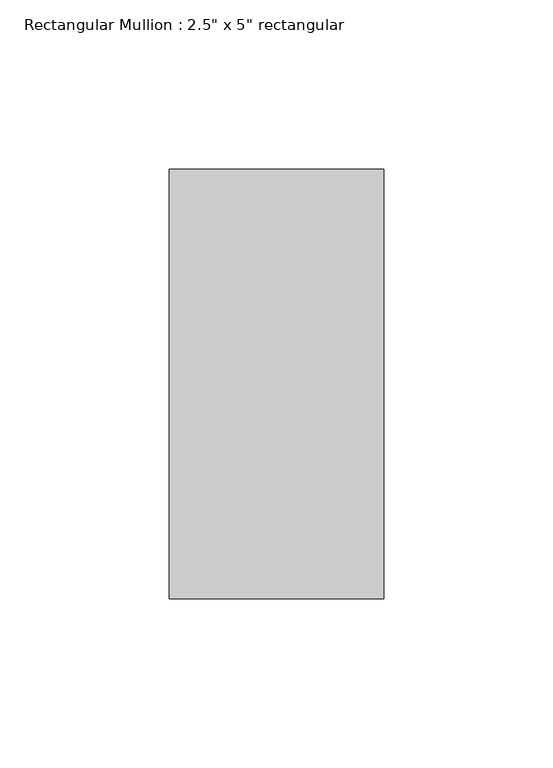
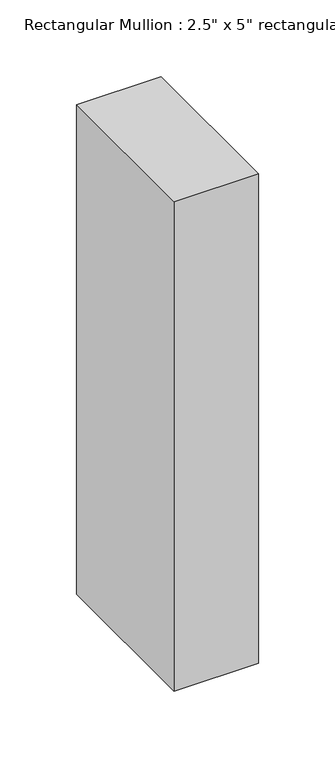
"""IFC4 building model written with IfcOpenShell, lengths in millimetres: member geometry."""

from ifc_helpers import new_model, si_unit, frame, origin, place, context, project, spatial, polyline, outline, extrude, source, transform, mapped, element, save


def member_de12f0f3(model_context):
    return source(origin(), model_context, "Body", "SweptSolid", [
        extrude(outline(polyline([(0.0, 63.5), (0.0, -63.5), (-63.5, -63.5), (-63.5, 63.5), (0.0, 63.5)])), frame((0.0, 0.0, -389.4666667), z_axis=(0.0, 0.0, 1.0), x_axis=(1.0, 0.0, 0.0)), (0.0, 0.0, 1.0), 389.4666667),
    ])


if __name__ == "__main__":
    model = new_model("IFC4")
    model_context = context("Model", 3, world=origin())
    ifc_project = project(units=[si_unit("LENGTHUNIT", "METRE", prefix="MILLI")], contexts=[model_context])
    site = spatial("IfcSite", under=ifc_project)
    building = spatial("IfcBuilding", under=site)
    placement = place(None, origin())
    member_shape = member_de12f0f3(model_context)
    element("IfcMember", 1, ObjectType="Rectangular Mullion : 2.5\" x 5\" rectangular", at=placement, inside=building, context=model_context, shape_type="MappedRepresentation", body=[
        mapped(member_shape, transform((0.0, 0.0, 0.0), x_axis=(1.0, 0.0, 0.0), y_axis=(0.0, 1.0, 0.0), z_axis=(0.0, 0.0, 1.0))),
    ])
    save(model, "model.ifc")

# Revit data of these elements
# Type "Rectangular Mullion : 2.5\" x 5\" rectangular"
#   built-in parameter 1007304 = 0.416667 (stored number, unit not read)
#   built-in parameter 1007301 = 0.104167 (stored number, unit not read)
#   built-in parameter 1007300 = 0.104167 (stored number, unit not read)
# Element 1 (IfcMember, "Rectangular Mullion : 2.5\" x 5\" rectangular")
#   Materials on its faces: "Aluminum"
# Materials
#   "Aluminum": class "Metal", colour RGB 247 247 247, transparency 0, Description = "Aluminum 6061", Cost = 0
